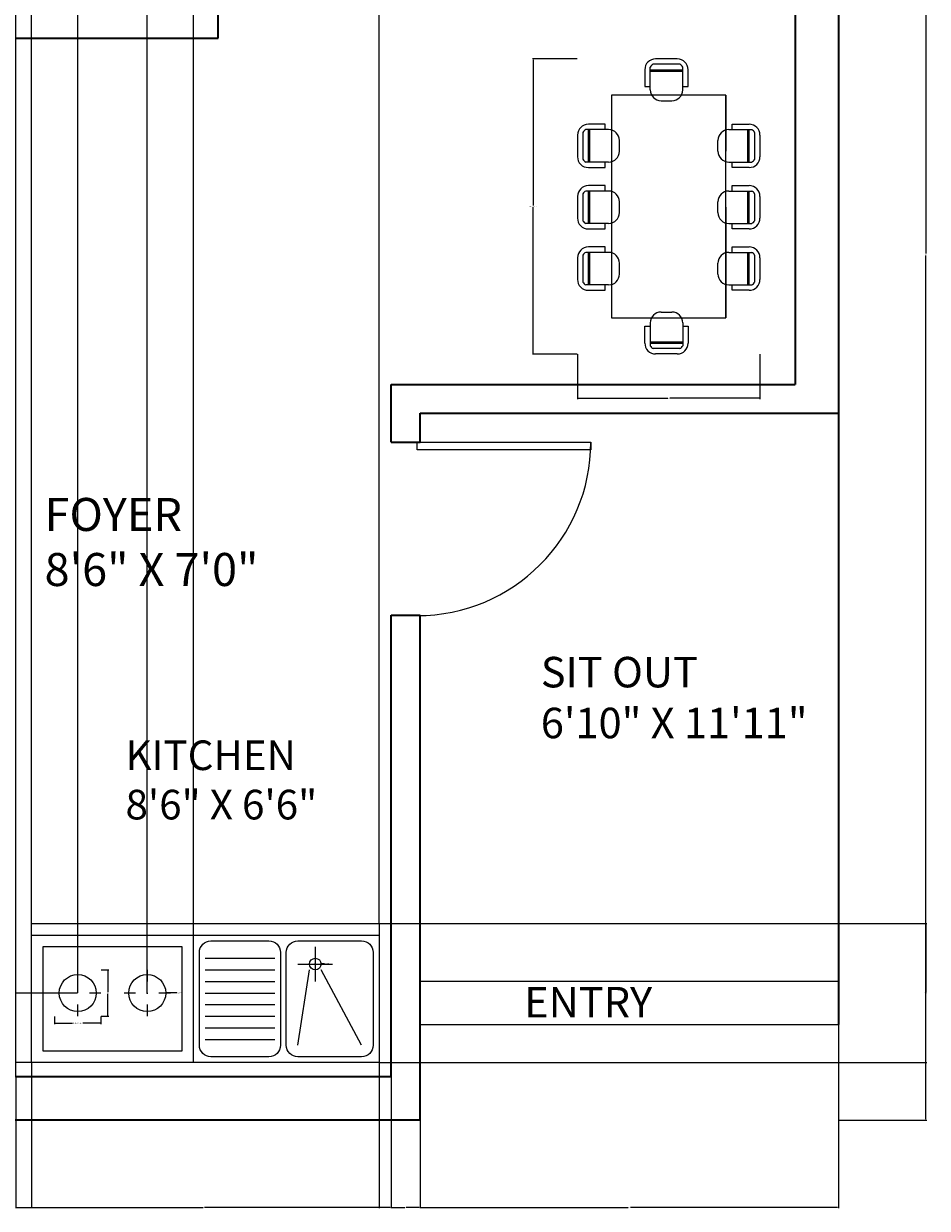
# Model space of a CAD drawing. Units: inches. Extents: x 2360 to 2721, y 1697 to 2094.
# Tile 2 of 3: x 2533 to 2721, y 1697 to 1944. Entities that reach past the tile are written whole.
import ezdxf

# ---------------------------------------------------------------- set-up
doc = ezdxf.new("R2010")
doc.units = ezdxf.units.IN
for name, color, linetype, lineweight in [('A-ANNO-DIMS', 2, 'Continuous', 18), ('A-AREA-IDEN', 7, 'Continuous', 18), ('A-DOOR', 4, 'Continuous', 25), ('A-EQPM', 42, 'Continuous', 18), ('A-FLOR-FIXT', 42, 'Continuous', 18), ('A-FLOR-STRS', 8, 'Continuous', 25), ('A-WALL', 7, 'Continuous', 35), ('FUR', 42, 'Continuous', 18)]:
    doc.layers.add(name, color=color, linetype=linetype, lineweight=lineweight)
doc.layers.add('TEFRIŞ', color=11, linetype='Continuous')
doc.styles.get("Standard").update_dxf_attribs({"font": 'arial.ttf'})
doc.dimstyles.get("Standard").update_dxf_attribs({"dimtxt": 0.18, "dimasz": 0.18, "dimexe": 0.18, "dimexo": 0.0625, "dimgap": 0.09, "dimtad": 0, "dimtih": 1, "dimtoh": 1, "dimdec": 4, "dimzin": 0, "dimdsep": 46, "dimtxsty": 'Standard', "dimcen": 0.09, "dimadec": 0, "dimazin": 0, "dimtfac": 1, "dimtdec": 4, "dimtofl": 0, "dimtmove": 0, "dimatfit": 3, "dimfxl": 1, "dimtolj": 1, "dimtzin": 0, "dimarcsym": 0})

# ---------------------------------------------------------------- blocks, each defined once
blk = doc.blocks.new('*U4')
for p, q in [((-40, 0), (-40, 6)), ((0, 0), (0, 6))]:
    blk.add_line(p, q)
blk.add_lwpolyline([(0, 0), (0, -40), (-1.75, -40), (-1.75, 0)], close=True)
blk.add_arc((0, 0), 40, 180, 270)
blk = doc.blocks.new('16')
at = {"layer": 'TEFRIŞ'}
for p, q in [((-1595.55, 335.61), (-1573.17, 335.61)), ((-1593.36, 340.11), (-1575.37, 340.11)), ((-1544.52, 335.61), (-1522.14, 335.61)), ((-1542.32, 340.11), (-1524.33, 340.11)), ((-1493.48, 335.61), (-1471.11, 335.61)), ((-1491.29, 340.11), (-1473.3, 340.11)), ((-1602.38, 316.98), (-1602.38, 331.09)), ((-1597.87, 314.22), (-1597.87, 333.28)), ((-1570.85, 331.1), (-1597.87, 331.1)), ((-1570.85, 329.98), (-1597.87, 329.98)), ((-1570.85, 314.22), (-1570.85, 333.28)), ((-1566.34, 331.09), (-1566.34, 316.98)), ((-1551.34, 316.98), (-1551.34, 331.09)), ((-1546.84, 314.22), (-1546.84, 333.28)), ((-1519.82, 331.1), (-1546.84, 331.1)), ((-1519.82, 329.98), (-1546.84, 329.98)), ((-1519.82, 314.22), (-1519.82, 333.28)), ((-1515.31, 331.09), (-1515.31, 316.98)), ((-1500.31, 316.98), (-1500.31, 331.09)), ((-1495.81, 314.22), (-1495.81, 333.28)), ((-1468.78, 331.1), (-1495.81, 331.1)), ((-1468.78, 329.98), (-1495.81, 329.98)), ((-1468.78, 314.22), (-1468.78, 333.28)), ((-1464.28, 331.09), (-1464.28, 316.98)), ((-1597.87, 316.98), (-1602.38, 316.98)), ((-1566.34, 316.98), (-1570.85, 316.98)), ((-1546.84, 316.98), (-1551.34, 316.98)), ((-1515.31, 316.98), (-1519.82, 316.98)), ((-1495.81, 316.98), (-1500.31, 316.98)), ((-1464.28, 316.98), (-1468.78, 316.98)), ((-1441.5, 311.75), (-1626.5, 311.75)), ((-1626.5, 311.75), (-1626.5, 216.75)), ((-1626.5, 311.75), (-1579.91, 311.75)), ((-1533.33, 311.75), (-1626.5, 311.75)), ((-1533.33, 311.75), (-1441.5, 311.75)), ((-1441.5, 216.75), (-1441.5, 311.75)), ((-1579.87, 305.2), (-1588.85, 305.2)), ((-1528.84, 305.2), (-1537.82, 305.2)), ((-1477.8, 305.2), (-1486.79, 305.2)), ((-1630.86, 275.89), (-1649.91, 275.89)), ((-1647.73, 248.86), (-1647.73, 275.89)), ((-1633.61, 280.39), (-1647.72, 280.39)), ((-1646.61, 248.86), (-1646.61, 275.89)), ((-1633.61, 275.89), (-1633.61, 280.39)), ((-1437.18, 275.89), (-1418.13, 275.89)), ((-1434.43, 275.89), (-1434.43, 280.39)), ((-1434.43, 280.39), (-1420.32, 280.39)), ((-1421.43, 248.86), (-1421.43, 275.89)), ((-1420.31, 248.86), (-1420.31, 275.89)), ((-1656.74, 271.37), (-1656.74, 253.38)), ((-1652.24, 273.57), (-1652.24, 251.19)), ((-1621.83, 257.89), (-1621.83, 266.87)), ((-1446.2, 257.89), (-1446.2, 266.87)), ((-1415.8, 273.57), (-1415.8, 251.19)), ((-1411.3, 271.37), (-1411.3, 253.38)), ((-1630.86, 248.86), (-1649.91, 248.86)), ((-1633.61, 244.36), (-1633.61, 248.86)), ((-1437.18, 248.86), (-1418.13, 248.86)), ((-1434.43, 244.36), (-1434.43, 248.86)), ((-1647.72, 244.36), (-1633.61, 244.36)), ((-1420.32, 244.36), (-1434.43, 244.36)), ((-1626.5, 216.75), (-1441.5, 216.75)), ((-1579.87, 223.3), (-1588.85, 223.3)), ((-1528.84, 223.3), (-1537.82, 223.3)), ((-1477.8, 223.3), (-1486.79, 223.3)), ((-1602.38, 211.53), (-1602.38, 197.42)), ((-1597.87, 211.53), (-1602.38, 211.53)), ((-1597.87, 214.28), (-1597.87, 195.23)), ((-1570.85, 214.28), (-1570.85, 195.23)), ((-1566.34, 211.53), (-1570.85, 211.53)), ((-1566.34, 197.42), (-1566.34, 211.53)), ((-1551.34, 211.53), (-1551.34, 197.42)), ((-1546.84, 211.53), (-1551.34, 211.53)), ((-1546.84, 214.28), (-1546.84, 195.23)), ((-1519.82, 214.28), (-1519.82, 195.23)), ((-1515.31, 211.53), (-1519.82, 211.53)), ((-1515.31, 197.42), (-1515.31, 211.53)), ((-1500.31, 211.53), (-1500.31, 197.42)), ((-1495.81, 211.53), (-1500.31, 211.53)), ((-1495.81, 214.28), (-1495.81, 195.23)), ((-1468.78, 214.28), (-1468.78, 195.23)), ((-1464.28, 211.53), (-1468.78, 211.53)), ((-1464.28, 197.42), (-1464.28, 211.53)), ((-1570.85, 198.53), (-1597.87, 198.53)), ((-1570.85, 197.41), (-1597.87, 197.41)), ((-1519.82, 198.53), (-1546.84, 198.53)), ((-1519.82, 197.41), (-1546.84, 197.41)), ((-1468.78, 198.53), (-1495.81, 198.53)), ((-1468.78, 197.41), (-1495.81, 197.41)), ((-1595.55, 192.9), (-1573.17, 192.9)), ((-1593.36, 188.4), (-1575.37, 188.4)), ((-1544.52, 192.9), (-1522.14, 192.9)), ((-1542.32, 188.4), (-1524.33, 188.4)), ((-1493.48, 192.9), (-1471.11, 192.9)), ((-1491.29, 188.4), (-1473.3, 188.4))]:
    blk.add_line(p, q, dxfattribs=at)
for centre, radius, start, end in [((-1593.36, 331.09), 9.02, 90, 180), ((-1593.36, 331.09), 5.02, 115.89448, 154.10552), ((-1575.37, 331.09), 9.02, 0, 90), ((-1575.37, 331.09), 5.02, 25.89448, 64.10552), ((-1542.32, 331.09), 9.02, 90, 180), ((-1542.32, 331.09), 5.02, 115.89448, 154.10552), ((-1524.33, 331.09), 9.02, 0, 90), ((-1524.33, 331.09), 5.02, 25.89448, 64.10552), ((-1491.29, 331.09), 9.02, 90, 180), ((-1491.29, 331.09), 5.02, 115.89448, 154.10552), ((-1473.3, 331.09), 9.02, 0, 90), ((-1473.3, 331.09), 5.02, 25.89448, 64.10552), ((-1588.85, 314.22), 9.02, 180, 270), ((-1579.87, 314.22), 9.02, 270, 0), ((-1537.82, 314.22), 9.02, 180, 270), ((-1528.84, 314.22), 9.02, 270, 0), ((-1486.79, 314.22), 9.02, 180, 270), ((-1477.8, 314.22), 9.02, 270, 0), ((-1647.72, 271.37), 9.02, 90, 180), ((-1647.72, 271.37), 5.02, 115.89448, 154.10552), ((-1630.86, 266.87), 9.02, 0, 90), ((-1437.18, 266.87), 9.02, 90, 180), ((-1420.32, 271.37), 9.02, 0, 90), ((-1420.32, 271.37), 5.02, 25.89448, 64.10552), ((-1630.86, 257.89), 9.02, 270, 0), ((-1437.18, 257.89), 9.02, 180, 270), ((-1647.72, 253.38), 9.02, 180, 270), ((-1647.72, 253.38), 5.02, 205.89448, 244.10552), ((-1420.32, 253.38), 9.02, 270, 0), ((-1420.32, 253.38), 5.02, 295.89448, 334.10552), ((-1588.85, 214.28), 9.02, 90, 180), ((-1579.87, 214.28), 9.02, 0, 90), ((-1537.82, 214.28), 9.02, 90, 180), ((-1528.84, 214.28), 9.02, 0, 90), ((-1486.79, 214.28), 9.02, 90, 180), ((-1477.8, 214.28), 9.02, 0, 90), ((-1593.36, 197.42), 9.02, 180, 270), ((-1575.37, 197.42), 9.02, 270, 0), ((-1542.32, 197.42), 9.02, 180, 270), ((-1524.33, 197.42), 9.02, 270, 0), ((-1491.29, 197.42), 9.02, 180, 270), ((-1473.3, 197.42), 9.02, 270, 0), ((-1593.36, 197.42), 5.02, 205.89448, 244.10552), ((-1575.37, 197.42), 5.02, 295.89448, 334.10552), ((-1542.32, 197.42), 5.02, 205.89448, 244.10552), ((-1524.33, 197.42), 5.02, 295.89448, 334.10552), ((-1491.29, 197.42), 5.02, 205.89448, 244.10552), ((-1473.3, 197.42), 5.02, 295.89448, 334.10552)]:
    blk.add_arc(centre, radius, start, end, dxfattribs=at)
blk = doc.blocks.new('COOKTOP-BURNER')
for p, q in [((4.82, 7.23), (4.82, 9.64)), ((2.41, 4.82), (0, 4.82)), ((9.64, 4.82), (7.23, 4.82)), ((4.82, 0), (4.82, 2.41))]:
    blk.add_line(p, q)
blk.add_circle((4.82, 4.82), 3.85)
blk = doc.blocks.new('*D13')
at = {"layer": 'A-ANNO-DIMS', "color": 0, "lineweight": -2, "transparency": 16777216}
for p, q in [((2539.65, 1737.2), (2539.65, 1735.64)), ((2549.28, 1737.2), (2549.28, 1735.64)), ((2539.83, 1735.82), (2543.38, 1735.82)), ((2549.1, 1735.82), (2545.56, 1735.82))]:
    blk.add_line(p, q, dxfattribs=at)
at = {"layer": 'A-ANNO-DIMS', "color": 0, "transparency": 16777216}
for points in [[(2539.83, 1735.85), (2539.83, 1735.79), (2539.65, 1735.82)], [(2549.1, 1735.85), (2549.1, 1735.79), (2549.28, 1735.82)]]:
    blk.add_solid(points, dxfattribs=at)
at = {"layer": 'Defpoints', "color": 0, "transparency": 16777216}
for p in [(2539.65, 1737.26), (2549.28, 1737.26), (2549.28, 1735.82)]:
    blk.add_point(p, dxfattribs=at)
at = {"layer": 'A-ANNO-DIMS', "color": 0, "transparency": 16777216, "insert": (2544.47, 1735.82), "char_height": 0.18, "attachment_point": 5}
blk.add_mtext('\\A1;BURNER 10 TYP.', dxfattribs=at)
blk = doc.blocks.new('*D14')
at = {"layer": 'A-ANNO-DIMS', "color": 0, "lineweight": -2, "transparency": 16777216}
for p, q in [((2549.35, 1746.9), (2550.91, 1746.9)), ((2550.73, 1746.72), (2550.73, 1742.26)), ((2550.73, 1737.44), (2550.73, 1741.9)), ((2549.35, 1737.26), (2550.91, 1737.26))]:
    blk.add_line(p, q, dxfattribs=at)
at = {"layer": 'A-ANNO-DIMS', "color": 0, "transparency": 16777216}
for points in [[(2550.7, 1746.72), (2550.76, 1746.72), (2550.73, 1746.9)], [(2550.7, 1737.44), (2550.76, 1737.44), (2550.73, 1737.26)]]:
    blk.add_solid(points, dxfattribs=at)
at = {"layer": 'Defpoints', "color": 0, "transparency": 16777216}
for p in [(2549.28, 1746.9), (2550.73, 1746.9), (2549.28, 1737.26)]:
    blk.add_point(p, dxfattribs=at)
at = {"layer": 'A-ANNO-DIMS', "color": 0, "transparency": 16777216, "insert": (2550.73, 1742.08), "char_height": 0.18, "attachment_point": 5}
blk.add_mtext('\\A1;10 TYP.', dxfattribs=at)
blk = doc.blocks.new('*D15')
at = {"layer": 'A-ANNO-DIMS', "color": 0, "lineweight": -2, "transparency": 16777216}
for p, q in [((2648.3, 1936.34), (2638.98, 1936.34)), ((2639.16, 1936.16), (2639.16, 1905.83)), ((2639.16, 1875.14), (2639.16, 1905.47)), ((2648.3, 1874.96), (2638.98, 1874.96))]:
    blk.add_line(p, q, dxfattribs=at)
at = {"layer": 'A-ANNO-DIMS', "color": 0, "transparency": 16777216}
for points in [[(2639.13, 1936.16), (2639.19, 1936.16), (2639.16, 1936.34)], [(2639.13, 1875.14), (2639.19, 1875.14), (2639.16, 1874.96)]]:
    blk.add_solid(points, dxfattribs=at)
at = {"layer": 'Defpoints', "color": 0, "transparency": 16777216}
for p in [(2648.37, 1936.34), (2639.16, 1874.96), (2648.37, 1874.96)]:
    blk.add_point(p, dxfattribs=at)
at = {"layer": 'A-ANNO-DIMS', "color": 0, "transparency": 16777216, "insert": (2639.16, 1905.65), "char_height": 0.18, "attachment_point": 5}
blk.add_mtext('\\A1;DINING SET 61', dxfattribs=at)
blk = doc.blocks.new('*D16')
at = {"layer": 'A-ANNO-DIMS', "color": 0, "lineweight": -2, "transparency": 16777216}
for p, q in [((2648.37, 1874.9), (2648.37, 1865.58)), ((2686.3, 1874.9), (2686.3, 1865.58)), ((2648.55, 1865.76), (2667.12, 1865.76)), ((2686.12, 1865.76), (2667.55, 1865.76))]:
    blk.add_line(p, q, dxfattribs=at)
at = {"layer": 'A-ANNO-DIMS', "color": 0, "transparency": 16777216}
for points in [[(2648.55, 1865.79), (2648.55, 1865.73), (2648.37, 1865.76)], [(2686.12, 1865.79), (2686.12, 1865.73), (2686.3, 1865.76)]]:
    blk.add_solid(points, dxfattribs=at)
at = {"layer": 'Defpoints', "color": 0, "transparency": 16777216}
for p in [(2648.37, 1874.96), (2686.3, 1874.96), (2686.3, 1865.76)]:
    blk.add_point(p, dxfattribs=at)
at = {"layer": 'A-ANNO-DIMS', "color": 0, "transparency": 16777216, "insert": (2667.33, 1865.76), "char_height": 0.18, "attachment_point": 5}
blk.add_mtext('\\A1;38', dxfattribs=at)
blk = doc.blocks.new('*D18')
at = {"layer": 'A-ANNO-DIMS', "color": 0, "lineweight": -2, "transparency": 16777216}
for p, q in [((2702.69, 2075.65), (2720.96, 2075.65)), ((2720.78, 2075.47), (2720.78, 1895.83)), ((2720.78, 1715.83), (2720.78, 1895.46)), ((2702.69, 1715.65), (2720.96, 1715.65))]:
    blk.add_line(p, q, dxfattribs=at)
at = {"layer": 'A-ANNO-DIMS', "color": 0, "transparency": 16777216}
for points in [[(2720.75, 2075.47), (2720.81, 2075.47), (2720.78, 2075.65)], [(2720.75, 1715.83), (2720.81, 1715.83), (2720.78, 1715.65)]]:
    blk.add_solid(points, dxfattribs=at)
at = {"layer": 'Defpoints', "color": 0, "transparency": 16777216}
for p in [(2702.63, 2075.65), (2720.78, 2075.65), (2702.63, 1715.65)]:
    blk.add_point(p, dxfattribs=at)
at = {"layer": 'A-ANNO-DIMS', "color": 0, "transparency": 16777216, "insert": (2720.78, 1895.65), "char_height": 0.18, "attachment_point": 5}
blk.add_mtext('\\A1;360', dxfattribs=at)
blk = doc.blocks.new('*D21')
at = {"layer": 'A-ANNO-DIMS', "color": 0, "lineweight": -2, "transparency": 16777216}
for p, q in [((2531.63, 1724.58), (2531.63, 1697.32)), ((2609.63, 1724.58), (2609.63, 1697.32)), ((2531.81, 1697.5), (2570.41, 1697.5)), ((2609.45, 1697.5), (2570.85, 1697.5))]:
    blk.add_line(p, q, dxfattribs=at)
at = {"layer": 'A-ANNO-DIMS', "color": 0, "transparency": 16777216}
for points in [[(2531.81, 1697.53), (2531.81, 1697.47), (2531.63, 1697.5)], [(2609.45, 1697.53), (2609.45, 1697.47), (2609.63, 1697.5)]]:
    blk.add_solid(points, dxfattribs=at)
at = {"layer": 'Defpoints', "color": 0, "transparency": 16777216}
for p in [(2531.63, 1724.65), (2609.63, 1724.65), (2609.63, 1697.5)]:
    blk.add_point(p, dxfattribs=at)
at = {"layer": 'A-ANNO-DIMS', "color": 0, "transparency": 16777216, "insert": (2570.63, 1697.5), "char_height": 0.18, "attachment_point": 5}
blk.add_mtext('\\A1;78', dxfattribs=at)
blk = doc.blocks.new('*D22')
at = {"layer": 'A-ANNO-DIMS', "color": 0, "lineweight": -2, "transparency": 16777216}
for p, q in [((2609.63, 1724.58), (2609.63, 1697.32)), ((2615.63, 1715.58), (2615.63, 1697.32)), ((2609.81, 1697.5), (2612.48, 1697.5)), ((2615.45, 1697.5), (2612.78, 1697.5))]:
    blk.add_line(p, q, dxfattribs=at)
at = {"layer": 'A-ANNO-DIMS', "color": 0, "transparency": 16777216}
for points in [[(2609.81, 1697.53), (2609.81, 1697.47), (2609.63, 1697.5)], [(2615.45, 1697.53), (2615.45, 1697.47), (2615.63, 1697.5)]]:
    blk.add_solid(points, dxfattribs=at)
at = {"layer": 'Defpoints', "color": 0, "transparency": 16777216}
for p in [(2609.63, 1724.65), (2615.63, 1715.65), (2615.63, 1697.5)]:
    blk.add_point(p, dxfattribs=at)
at = {"layer": 'A-ANNO-DIMS', "color": 0, "transparency": 16777216, "insert": (2612.63, 1697.5), "char_height": 0.18, "attachment_point": 5}
blk.add_mtext('\\A1;6', dxfattribs=at)
blk = doc.blocks.new('*D23')
at = {"layer": 'A-ANNO-DIMS', "color": 0, "lineweight": -2, "transparency": 16777216}
for p, q in [((2615.63, 1715.58), (2615.63, 1697.32)), ((2702.63, 1715.58), (2702.63, 1697.32)), ((2615.81, 1697.5), (2658.91, 1697.5)), ((2702.45, 1697.5), (2659.35, 1697.5))]:
    blk.add_line(p, q, dxfattribs=at)
at = {"layer": 'A-ANNO-DIMS', "color": 0, "transparency": 16777216}
for points in [[(2615.81, 1697.53), (2615.81, 1697.47), (2615.63, 1697.5)], [(2702.45, 1697.53), (2702.45, 1697.47), (2702.63, 1697.5)]]:
    blk.add_solid(points, dxfattribs=at)
at = {"layer": 'Defpoints', "color": 0, "transparency": 16777216}
for p in [(2615.63, 1715.65), (2702.63, 1715.65), (2702.63, 1697.5)]:
    blk.add_point(p, dxfattribs=at)
at = {"layer": 'A-ANNO-DIMS', "color": 0, "transparency": 16777216, "insert": (2659.13, 1697.5), "char_height": 0.18, "attachment_point": 5}
blk.add_mtext('\\A1;87', dxfattribs=at)
blk = doc.blocks.new('*D31')
at = {"layer": 'A-ANNO-DIMS', "color": 0, "lineweight": -2, "transparency": 16777216}
for p, q in [((2534.83, 1727.56), (2534.83, 1697.32)), ((2607.1, 1727.56), (2607.1, 1697.32)), ((2535.01, 1697.5), (2570.57, 1697.5)), ((2606.92, 1697.5), (2571.36, 1697.5))]:
    blk.add_line(p, q, dxfattribs=at)
at = {"layer": 'A-ANNO-DIMS', "color": 0, "transparency": 16777216}
for points in [[(2535.01, 1697.53), (2535.01, 1697.47), (2534.83, 1697.5)], [(2606.92, 1697.53), (2606.92, 1697.47), (2607.1, 1697.5)]]:
    blk.add_solid(points, dxfattribs=at)
at = {"layer": 'Defpoints', "color": 0, "transparency": 16777216}
for p in [(2534.83, 1727.63), (2607.1, 1727.63), (2607.1, 1697.5)]:
    blk.add_point(p, dxfattribs=at)
at = {"layer": 'A-ANNO-DIMS', "color": 0, "transparency": 16777216, "insert": (2570.97, 1697.5), "char_height": 0.18, "attachment_point": 5}
blk.add_mtext('\\A1;72.27', dxfattribs=at)
blk = doc.blocks.new('*D32')
at = {"layer": 'A-ANNO-DIMS', "color": 0, "lineweight": -2, "transparency": 16777216}
for p, q in [((2607.16, 1756.53), (2720.96, 1756.53)), ((2720.78, 1756.35), (2720.78, 1742.26)), ((2720.78, 1727.81), (2720.78, 1741.9)), ((2607.16, 1727.63), (2720.96, 1727.63))]:
    blk.add_line(p, q, dxfattribs=at)
at = {"layer": 'A-ANNO-DIMS', "color": 0, "transparency": 16777216}
for points in [[(2720.75, 1756.35), (2720.81, 1756.35), (2720.78, 1756.53)], [(2720.75, 1727.81), (2720.81, 1727.81), (2720.78, 1727.63)]]:
    blk.add_solid(points, dxfattribs=at)
at = {"layer": 'Defpoints', "color": 0, "transparency": 16777216}
for p in [(2607.1, 1756.53), (2720.78, 1756.53), (2607.1, 1727.63)]:
    blk.add_point(p, dxfattribs=at)
at = {"layer": 'A-ANNO-DIMS', "color": 0, "transparency": 16777216, "insert": (2720.78, 1742.08), "char_height": 0.18, "attachment_point": 5}
blk.add_mtext('\\A1;28.91', dxfattribs=at)
blk = doc.blocks.new('*D33')
at = {"layer": 'A-ANNO-DIMS', "color": 0, "lineweight": -2, "transparency": 16777216}
for p, q in [((2568.56, 1756.6), (2568.56, 2093.98)), ((2607.1, 1756.6), (2607.1, 2093.98)), ((2568.74, 2093.8), (2587.43, 2093.8)), ((2606.92, 2093.8), (2588.22, 2093.8))]:
    blk.add_line(p, q, dxfattribs=at)
at = {"layer": 'A-ANNO-DIMS', "color": 0, "transparency": 16777216}
for points in [[(2568.74, 2093.83), (2568.74, 2093.77), (2568.56, 2093.8)], [(2606.92, 2093.83), (2606.92, 2093.77), (2607.1, 2093.8)]]:
    blk.add_solid(points, dxfattribs=at)
at = {"layer": 'Defpoints', "color": 0, "transparency": 16777216}
for p in [(2607.1, 2093.8), (2568.56, 1756.53), (2607.1, 1756.53)]:
    blk.add_point(p, dxfattribs=at)
at = {"layer": 'A-ANNO-DIMS', "color": 0, "transparency": 16777216, "insert": (2587.83, 2093.8), "char_height": 0.18, "attachment_point": 5}
blk.add_mtext('\\A1;38.54', dxfattribs=at)
blk = doc.blocks.new('*D34')
at = {"layer": 'A-ANNO-DIMS', "color": 0, "lineweight": -2, "transparency": 16777216}
for p, q in [((2544.47, 1742.14), (2544.47, 2093.98)), ((2558.92, 1742.14), (2558.92, 2093.98)), ((2544.65, 2093.8), (2551.24, 2093.8)), ((2558.74, 2093.8), (2552.15, 2093.8))]:
    blk.add_line(p, q, dxfattribs=at)
at = {"layer": 'A-ANNO-DIMS', "color": 0, "transparency": 16777216}
for points in [[(2544.65, 2093.83), (2544.65, 2093.77), (2544.47, 2093.8)], [(2558.74, 2093.83), (2558.74, 2093.77), (2558.92, 2093.8)]]:
    blk.add_solid(points, dxfattribs=at)
at = {"layer": 'Defpoints', "color": 0, "transparency": 16777216}
for p in [(2558.92, 2093.8), (2544.47, 1742.08), (2558.92, 1742.08)]:
    blk.add_point(p, dxfattribs=at)
at = {"layer": 'A-ANNO-DIMS', "color": 0, "transparency": 16777216, "insert": (2551.69, 2093.8), "char_height": 0.18, "attachment_point": 5}
blk.add_mtext('\\A1;14.454', dxfattribs=at)
blk = doc.blocks.new('*D35')
at = {"layer": 'A-ANNO-DIMS', "color": 0, "lineweight": -2, "transparency": 16777216}
for p, q in [((2534.83, 1727.69), (2534.83, 2093.98)), ((2544.47, 1742.14), (2544.47, 2093.98)), ((2535.01, 2093.8), (2539.25, 2093.8)), ((2544.29, 2093.8), (2540.04, 2093.8))]:
    blk.add_line(p, q, dxfattribs=at)
at = {"layer": 'A-ANNO-DIMS', "color": 0, "transparency": 16777216}
for points in [[(2535.01, 2093.83), (2535.01, 2093.77), (2534.83, 2093.8)], [(2544.29, 2093.83), (2544.29, 2093.77), (2544.47, 2093.8)]]:
    blk.add_solid(points, dxfattribs=at)
at = {"layer": 'Defpoints', "color": 0, "transparency": 16777216}
for p in [(2544.47, 2093.8), (2544.47, 1742.08), (2534.83, 1727.63)]:
    blk.add_point(p, dxfattribs=at)
at = {"layer": 'A-ANNO-DIMS', "color": 0, "transparency": 16777216, "insert": (2539.65, 2093.8), "char_height": 0.18, "attachment_point": 5}
blk.add_mtext('\\A1;9.636', dxfattribs=at)
blk = doc.blocks.new('*D36')
at = {"layer": 'A-ANNO-DIMS', "color": 0, "lineweight": -2, "transparency": 16777216}
for p, q in [((2544.4, 1742.08), (2360.3, 1742.08)), ((2360.48, 1741.9), (2360.48, 1735.04)), ((2360.48, 1727.81), (2360.48, 1734.67)), ((2534.77, 1727.63), (2360.3, 1727.63))]:
    blk.add_line(p, q, dxfattribs=at)
at = {"layer": 'A-ANNO-DIMS', "color": 0, "transparency": 16777216}
for points in [[(2360.45, 1741.9), (2360.51, 1741.9), (2360.48, 1742.08)], [(2360.45, 1727.81), (2360.51, 1727.81), (2360.48, 1727.63)]]:
    blk.add_solid(points, dxfattribs=at)
at = {"layer": 'Defpoints', "color": 0, "transparency": 16777216}
for p in [(2360.48, 1742.08), (2544.47, 1742.08), (2534.83, 1727.63)]:
    blk.add_point(p, dxfattribs=at)
at = {"layer": 'A-ANNO-DIMS', "color": 0, "transparency": 16777216, "insert": (2360.48, 1734.85), "char_height": 0.18, "attachment_point": 5}
blk.add_mtext('\\A1;14.454', dxfattribs=at)
blk = doc.blocks.new('*D37')
at = {"layer": 'A-ANNO-DIMS', "color": 0, "lineweight": -2, "transparency": 16777216}
for p, q in [((2531.63, 1724.71), (2531.63, 2093.98)), ((2534.83, 1727.69), (2534.83, 2093.98)), ((2531.81, 2093.8), (2532.84, 2093.8)), ((2534.65, 2093.8), (2533.63, 2093.8))]:
    blk.add_line(p, q, dxfattribs=at)
at = {"layer": 'A-ANNO-DIMS', "color": 0, "transparency": 16777216}
for points in [[(2531.81, 2093.83), (2531.81, 2093.77), (2531.63, 2093.8)], [(2534.65, 2093.83), (2534.65, 2093.77), (2534.83, 2093.8)]]:
    blk.add_solid(points, dxfattribs=at)
at = {"layer": 'Defpoints', "color": 0, "transparency": 16777216}
for p in [(2534.83, 2093.8), (2534.83, 1727.63), (2531.63, 1724.65)]:
    blk.add_point(p, dxfattribs=at)
at = {"layer": 'A-ANNO-DIMS', "color": 0, "transparency": 16777216, "insert": (2533.23, 2093.8), "char_height": 0.18, "attachment_point": 5}
blk.add_mtext('\\A1;3.198', dxfattribs=at)
blk = doc.blocks.new('*D38')
at = {"layer": 'A-ANNO-DIMS', "color": 0, "lineweight": -2, "transparency": 16777216}
for p, q in [((2534.77, 1727.63), (2360.3, 1727.63)), ((2360.48, 1727.45), (2360.48, 1726.32)), ((2531.57, 1724.65), (2360.3, 1724.65)), ((2360.48, 1724.83), (2360.48, 1725.95))]:
    blk.add_line(p, q, dxfattribs=at)
at = {"layer": 'A-ANNO-DIMS', "color": 0, "transparency": 16777216}
for points in [[(2360.45, 1727.45), (2360.51, 1727.45), (2360.48, 1727.63)], [(2360.45, 1724.83), (2360.51, 1724.83), (2360.48, 1724.65)]]:
    blk.add_solid(points, dxfattribs=at)
at = {"layer": 'Defpoints', "color": 0, "transparency": 16777216}
for p in [(2360.48, 1727.63), (2534.83, 1727.63), (2531.63, 1724.65)]:
    blk.add_point(p, dxfattribs=at)
at = {"layer": 'A-ANNO-DIMS', "color": 0, "transparency": 16777216, "insert": (2360.48, 1726.14), "char_height": 0.18, "attachment_point": 5}
blk.add_mtext('\\A1;2.98', dxfattribs=at)
blk = doc.blocks.new('*D39')
at = {"layer": 'A-ANNO-DIMS', "color": 0, "lineweight": -2, "transparency": 16777216}
for p, q in [((2593.76, 1748.1), (2593.94, 1748.1)), ((2593.85, 1748.01), (2593.85, 1748.19)), ((2595.78, 1748.17), (2595.23, 1748.15))]:
    blk.add_line(p, q, dxfattribs=at)
at = {"layer": 'A-ANNO-DIMS', "color": 0, "transparency": 16777216}
blk.add_solid([(2595.23, 1748.18), (2595.23, 1748.12), (2595.05, 1748.15)], dxfattribs=at)
at = {"layer": 'Defpoints', "color": 0, "transparency": 16777216}
for p in [(2592.65, 1748.06), (2595.05, 1748.15)]:
    blk.add_point(p, dxfattribs=at)
at = {"layer": 'A-ANNO-DIMS', "color": 0, "transparency": 16777216, "insert": (2596.27, 1748.17), "char_height": 0.18, "attachment_point": 5}
blk.add_mtext('\\A1;∅2.409', dxfattribs=at)
blk = doc.blocks.new('*D40')
at = {"layer": 'A-ANNO-DIMS', "color": 0, "lineweight": -2, "transparency": 16777216}
for p, q in [((2558.83, 1742.08), (2559.01, 1742.08)), ((2558.92, 1741.99), (2558.92, 1742.17)), ((2565.09, 1742.11), (2562.95, 1742.1))]:
    blk.add_line(p, q, dxfattribs=at)
at = {"layer": 'A-ANNO-DIMS', "color": 0, "transparency": 16777216}
blk.add_solid([(2562.95, 1742.13), (2562.95, 1742.07), (2562.77, 1742.1)], dxfattribs=at)
at = {"layer": 'Defpoints', "color": 0, "transparency": 16777216}
for p in [(2555.07, 1742.06), (2562.77, 1742.1)]:
    blk.add_point(p, dxfattribs=at)
at = {"layer": 'A-ANNO-DIMS', "color": 0, "transparency": 16777216, "insert": (2565.77, 1742.11), "char_height": 0.18, "attachment_point": 5}
blk.add_mtext('\\A1;2X ∅7.709', dxfattribs=at)

msp = doc.modelspace()

# ---------------------------------------------------------------- linework, layer by layer
at = {"layer": 'A-EQPM'}
msp.add_lwpolyline([(2566.1471, 1730.0357), (2566.1471, 1751.7165), (2537.2395, 1751.7165), (2537.2395, 1730.0357)], close=True, dxfattribs=at)
at = {"layer": 'A-FLOR-FIXT'}
for p, q in [((2568.5561, 1727.6267), (2568.5561, 1756.5344)), ((2534.8305, 1754.1254), (2607.0997, 1754.1254)), ((2593.8503, 1751.7165), (2593.8503, 1744.4895)), ((2570.9651, 1749.3075), (2585.4189, 1749.3075)), ((2570.9651, 1746.8985), (2585.4189, 1746.8985)), ((2590.2369, 1748.103), (2597.4638, 1748.103)), ((2590.2369, 1731.2402), (2592.6458, 1746.8985)), ((2603.4862, 1731.2402), (2595.0548, 1746.8985)), ((2570.9651, 1744.4895), (2585.4189, 1744.4895)), ((2570.9651, 1742.0806), (2585.4189, 1742.0806)), ((2570.9651, 1739.6716), (2585.4189, 1739.6716)), ((2570.9651, 1737.2626), (2585.4189, 1737.2626)), ((2570.9651, 1734.8537), (2585.4189, 1734.8537)), ((2570.9651, 1732.4447), (2585.4189, 1732.4447))]:
    msp.add_line(p, q, dxfattribs=at)
msp.add_lwpolyline([(2534.8305, 1756.5344), (2607.0997, 1756.5344), (2607.0997, 1727.6267), (2534.8305, 1727.6267)], close=True, dxfattribs=at)
for points in [[(2572.1696, 1752.9209), (2584.2144, 1752.9209, -0.41421356), (2586.6234, 1750.512), (2586.6234, 1731.2402, -0.41421356), (2584.2144, 1728.8312), (2572.1696, 1728.8312, -0.41421356), (2569.7606, 1731.2402), (2569.7606, 1750.512, -0.41421356)], [(2590.2369, 1752.9209), (2603.4862, 1752.9209, -0.41421356), (2605.8952, 1750.512), (2605.8952, 1731.2402, -0.41421356), (2603.4862, 1728.8312), (2590.2369, 1728.8312, -0.41421356), (2587.8279, 1731.2402), (2587.8279, 1750.512, -0.41421356)]]:
    msp.add_lwpolyline(points, format="xyb", close=True, dxfattribs=at)
msp.add_circle((2593.8503, 1748.103), 1.2045, dxfattribs=at)
at = {"layer": 'A-FLOR-STRS'}
for p, q in [((2615.6324, 1744.5718), (2702.6324, 1744.5718)), ((2615.6324, 1735.5718), (2702.6324, 1735.5718)), ((2702.6324, 1735.5718), (2702.6324, 1715.6468))]:
    msp.add_line(p, q, dxfattribs=at)
at = {"layer": 'A-WALL'}
for p, q in [((2702.6324, 2075.6468), (2702.6324, 1735.5718)), ((2693.6324, 2066.6468), (2693.6324, 1868.6468)), ((2573.6324, 1940.6468), (2573.6324, 1952.6468)), ((2441.6324, 1940.6468), (2561.6324, 1940.6468)), ((2561.6324, 1940.6468), (2573.6324, 1940.6468)), ((2609.6324, 1856.6468), (2609.6324, 1868.6468)), ((2609.6324, 1868.6468), (2693.6324, 1868.6468)), ((2615.6324, 1856.6468), (2615.6324, 1862.6468)), ((2615.6324, 1862.6468), (2702.6324, 1862.6468)), ((2609.6324, 1856.6468), (2615.6324, 1856.6468)), ((2609.6324, 1724.6468), (2609.6324, 1820.6468)), ((2609.6324, 1820.6468), (2615.6324, 1820.6468)), ((2615.6324, 1715.6468), (2615.6324, 1820.6468)), ((2609.6324, 1724.6468), (2531.6324, 1724.6468)), ((2615.6324, 1715.6468), (2378.6324, 1715.6468))]:
    msp.add_line(p, q, dxfattribs=at)

# ---------------------------------------------------------------- block references
at = {"layer": 'A-DOOR', "xscale": 0.9022924037583027, "yscale": 0.9022924037583027, "zscale": 0.9022924037583027, "rotation": 90}
msp.add_blockref('*U4', (2615.0461, 1856.6468), dxfattribs=at)
at = {"layer": 'A-EQPM'}
msp.add_blockref('COOKTOP-BURNER', (2539.648, 1737.263), dxfattribs=at)
at = {"layer": 'A-EQPM', "rotation": 89.99999999999731}
msp.add_blockref('COOKTOP-BURNER', (2563.7378, 1737.2622), dxfattribs=at)
at = {"layer": 'FUR', "xscale": 0.2500637396927753, "yscale": 0.2500637396927753, "zscale": 0.2500637396927753, "rotation": 270}
msp.add_blockref('16', (2601.2539, 1522.0475), dxfattribs=at)

# ---------------------------------------------------------------- texts
at = {"layer": 'A-AREA-IDEN', "attachment_point": 1}
for s, width, gutter_width, insert, char_height in [('FOYER \\P8\'6" X 7\'0"', 435.871112, 34.3312, (2537.5774, 1845.03), 6.866242), ('SIT OUT\\P6\'10" X 11\'11"', 402.638094, 31.7136, (2640.7339, 1811.9791), 6.342725), ('KITCHEN\\P8\'6" X 6\'6"', 390.91876, 30.7906, (2554.4002, 1794.6038), 6.158111), ('ENTRY', 402.638094, 31.7136, (2637.2718, 1743.3434), 6.34272)]:
    msp.add_mtext_dynamic_manual_height_columns(s, width=width, gutter_width=gutter_width, heights=[0], dxfattribs=dict(at, insert=insert, char_height=char_height))

# ---------------------------------------------------------------- dimensions: what is measured, and where the dimension line sits
at = {"layer": 'A-ANNO-DIMS'}
for base, p1, p2, override, picture, middle in [((2534.8305, 2093.7968), (2531.6324, 1724.6468), (2534.8305, 1727.6267), {"dimdec": 3, "dimlfac": 1, "dimrnd": 0, "dimzin": 0, "dimdsep": 46, "dimlunit": 2}, '*D37', (2533.2315, 2093.7968)), ((2544.4664, 2093.7968), (2534.8305, 1727.6267), (2544.4664, 1742.0806), {"dimdec": 3, "dimlfac": 1, "dimrnd": 0, "dimzin": 0, "dimdsep": 46, "dimlunit": 2}, '*D35', (2539.6485, 2093.7968)), ((2558.9202, 2093.7968), (2544.4664, 1742.0806), (2558.9202, 1742.0806), {"dimdec": 3, "dimlfac": 1, "dimrnd": 0, "dimzin": 0, "dimdsep": 46, "dimlunit": 2}, '*D34', (2551.6933, 2093.7968)), ((2607.0997, 2093.7968), (2568.5561, 1756.5344), (2607.0997, 1756.5344), {"dimdec": 2, "dimlfac": 1, "dimrnd": 0, "dimzin": 0, "dimdsep": 46, "dimlunit": 2}, '*D33', (2587.8279, 2093.7968)), ((2686.303, 1865.7554), (2648.3652, 1874.9619), (2686.303, 1874.9619), {"dimdec": 0, "dimlfac": 1, "dimrnd": 0, "dimzin": 0, "dimdsep": 46, "dimlunit": 2}, '*D16', (2667.3341, 1865.7554)), ((2607.0997, 1697.4968), (2534.8305, 1727.6267), (2607.0997, 1727.6267), {"dimdec": 2, "dimlfac": 1, "dimrnd": 0, "dimzin": 0, "dimdsep": 46, "dimlunit": 2}, '*D31', (2570.9651, 1697.4968)), ((2609.6324, 1697.4968), (2531.6324, 1724.6468), (2609.6324, 1724.6468), {"dimdec": 0, "dimlfac": 1, "dimrnd": 0, "dimzin": 0, "dimdsep": 46, "dimlunit": 2}, '*D21', (2570.6324, 1697.4968)), ((2615.6324, 1697.4968), (2609.6324, 1724.6468), (2615.6324, 1715.6468), {"dimdec": 0, "dimlfac": 1, "dimrnd": 0, "dimzin": 0, "dimdsep": 46, "dimlunit": 2}, '*D22', (2612.6324, 1697.4968)), ((2702.6324, 1697.4968), (2615.6324, 1715.6468), (2702.6324, 1715.6468), {"dimdec": 0, "dimlfac": 1, "dimrnd": 0, "dimzin": 0, "dimdsep": 46, "dimlunit": 2}, '*D23', (2659.1324, 1697.4968))]:
    dim = msp.add_linear_dim(base=base, p1=p1, p2=p2, dimstyle='Standard', override=override, dxfattribs=at)
    dim.commit()
    dim.dimension.update_dxf_attribs({"geometry": picture, "text_midpoint": middle})
for base, p1, p2, override, picture, middle in [((2720.7824, 2075.6468), (2702.6324, 1715.6468), (2702.6324, 2075.6468), {"dimdec": 0, "dimlfac": 1, "dimrnd": 0, "dimzin": 0, "dimdsep": 46, "dimlunit": 2}, '*D18', (2720.7824, 1895.6468)), ((2720.7824, 1756.5344), (2607.0997, 1727.6267), (2607.0997, 1756.5344), {"dimdec": 2, "dimlfac": 1, "dimrnd": 0, "dimzin": 0, "dimdsep": 46, "dimlunit": 2}, '*D32', (2720.7824, 1742.0806)), ((2360.4824, 1742.0806), (2534.8305, 1727.6267), (2544.4664, 1742.0806), {"dimdec": 3, "dimlfac": 1, "dimrnd": 0, "dimzin": 0, "dimdsep": 46, "dimlunit": 2}, '*D36', (2360.4824, 1734.8537)), ((2360.4824, 1727.6267), (2531.6324, 1724.6468), (2534.8305, 1727.6267), {"dimdec": 2, "dimlfac": 1, "dimrnd": 0, "dimzin": 0, "dimdsep": 46, "dimlunit": 2}, '*D38', (2360.4824, 1726.1368))]:
    dim = msp.add_linear_dim(base=base, p1=p1, p2=p2, angle=90, dimstyle='Standard', override=override, dxfattribs=at)
    dim.commit()
    dim.dimension.update_dxf_attribs({"geometry": picture, "text_midpoint": middle})
for base, p1, p2, angle, text, picture, middle in [((2639.1587, 1874.9619), (2648.3652, 1936.3384), (2648.3652, 1874.9619), 270, 'DINING SET <>', '*D15', (2639.1587, 1905.6501)), ((2550.7297, 1746.8985), (2549.2843, 1737.2626), (2549.2843, 1746.8985), 90, '<> TYP.', '*D14', (2550.7297, 1742.0806))]:
    dim = msp.add_linear_dim(base=base, p1=p1, p2=p2, angle=angle, text=text, dimstyle='Standard', override={"dimdec": 0, "dimlfac": 1, "dimrnd": 0, "dimzin": 0, "dimdsep": 46, "dimlunit": 2}, dxfattribs=at)
    dim.commit()
    dim.dimension.update_dxf_attribs({"geometry": picture, "text_midpoint": middle})
dim = msp.add_diameter_dim_2p(p1=(2592.6467, 1748.0585), p2=(2595.054, 1748.1476), dimstyle='Standard', override={"dimdec": 3, "dimlfac": 1, "dimrnd": 0, "dimzin": 0, "dimdsep": 46, "dimlunit": 2}, dxfattribs=at)
dim.commit()
dim.dimension.update_dxf_attribs({"geometry": '*D39', "text_midpoint": (2595.7762, 1748.1743), "dimtype": 163})
dim = msp.add_diameter_dim_2p(p1=(2555.0659, 1742.061), p2=(2562.7745, 1742.1001), text='2X <>', dimstyle='Standard', override={"dimdec": 3, "dimlfac": 1, "dimrnd": 0, "dimzin": 0, "dimdsep": 46, "dimlunit": 2}, dxfattribs=at)
dim.commit()
dim.dimension.update_dxf_attribs({"geometry": '*D40', "text_midpoint": (2565.0871, 1742.1119), "dimtype": 163})
dim = msp.add_linear_dim(base=(2549.2843, 1735.8173), p1=(2539.6485, 1737.2626), p2=(2549.2843, 1737.2626), text='BURNER <> TYP.', dimstyle='Standard', override={"dimdec": 0, "dimlfac": 1, "dimrnd": 0, "dimzin": 0, "dimdsep": 46, "dimlunit": 2}, dxfattribs=at)
dim.commit()
dim.dimension.update_dxf_attribs({"geometry": '*D13', "text_midpoint": (2544.4664, 1735.8173)})

doc.saveas('drawing.dxf')
